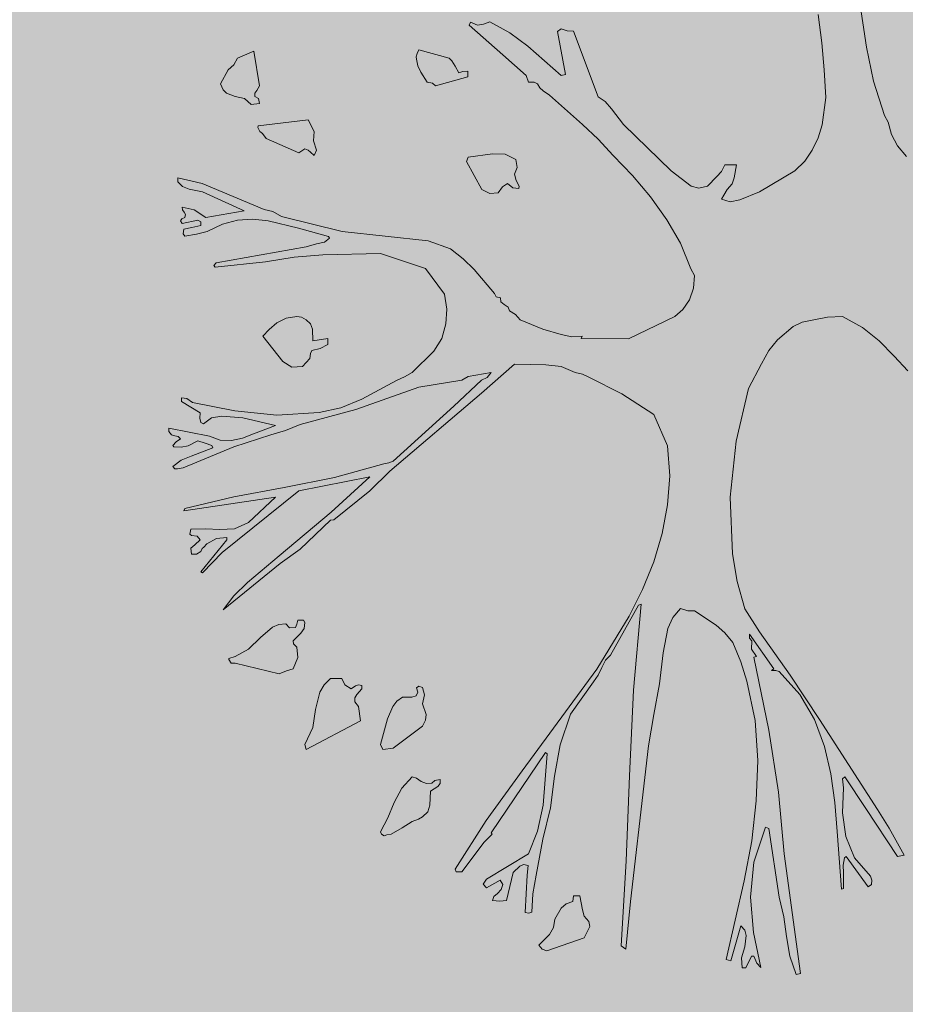
# Model space of a CAD drawing. Units: inches. Extents: x 84 to 1044, y -280 to 906.
# Tile 60 of 105: x 411.62 to 427.1, y 730.84 to 748.06. Entities that reach past the tile are written whole.
import ezdxf

# ---------------------------------------------------------------- set-up
doc = ezdxf.new("R2010")
doc.units = ezdxf.units.IN
doc.layers.add('A-ANNO-DIMS', color=2, linetype='Continuous', lineweight=18)
doc.layers.add('L-PLNT', color=114, linetype='Continuous', lineweight=15)
doc.layers.add('L-PLNT-PATT', color=9, linetype='Continuous', lineweight=9, true_color=0xafd9aa)
doc.styles.get("Standard").update_dxf_attribs({"font": 'arial.ttf'})
doc.dimstyles.get("Standard").update_dxf_attribs({"dimtxt": 0.18, "dimasz": 0.18, "dimexe": 0.18, "dimexo": 0.0625, "dimgap": 0.09, "dimtad": 0, "dimtih": 1, "dimtoh": 1, "dimdec": 4, "dimzin": 0, "dimdsep": 46, "dimtxsty": 'Standard', "dimcen": 0.09, "dimadec": 0, "dimazin": 0, "dimtfac": 1, "dimtdec": 4, "dimtofl": 0, "dimtmove": 0, "dimatfit": 3, "dimfxl": 1, "dimtolj": 1, "dimtzin": 0, "dimarcsym": 0})

# ---------------------------------------------------------------- blocks, each defined once
blk = doc.blocks.new('A$C37E508DF')
for p, q in [((0.7911, 1.1436), (0.8027, 1.0677)), ((0.7512, 1.0728), (0.7469, 1.1054)), ((0.3456, 1.093), (0.3469, 1.0964)), ((0.3842, 1.0591), (0.3456, 1.093)), ((0.3469, 1.0964), (0.355, 1.093)), ((0.355, 1.093), (0.3619, 1.0943)), ((0.3619, 1.0943), (0.3692, 1.0968)), ((0.3692, 1.0968), (0.3923, 1.0844)), ((0.4472, 1.0857), (0.4515, 1.0887)), ((0.4515, 1.0887), (0.4584, 1.0865)), ((0.3923, 1.0844), (0.4129, 1.069)), ((0.4562, 1.0364), (0.4472, 1.0857)), ((0.4584, 1.0865), (0.4657, 1.0861)), ((0.4657, 1.0861), (0.4939, 1.0107)), ((0.4129, 1.069), (0.4515, 1.0351)), ((0.7538, 1.0415), (0.7512, 1.0728)), ((0.8027, 1.0677), (0.8108, 1.0287)), ((0.0746, 1.0475), (0.0789, 1.0552)), ((0.0789, 1.0552), (0.0978, 1.063)), ((0.0978, 1.063), (0.1042, 1.0231)), ((0.2847, 1.0565), (0.2856, 1.0604)), ((0.2851, 1.054), (0.2847, 1.0565)), ((0.2856, 1.0604), (0.2877, 1.0647)), ((0.2877, 1.0647), (0.3224, 1.0552)), ((0.3224, 1.0552), (0.3255, 1.0522)), ((0.4112, 1.0351), (0.3842, 1.0591)), ((0.0682, 1.0415), (0.0746, 1.0475)), ((0.2864, 1.0463), (0.2851, 1.054)), ((0.2899, 1.039), (0.2864, 1.0463)), ((0.3255, 1.0522), (0.3293, 1.0458)), ((0.3293, 1.0458), (0.3336, 1.0381)), ((0.0596, 1.0257), (0.0682, 1.0415)), ((0.2972, 1.0274), (0.2899, 1.039)), ((0.3439, 1.0338), (0.3066, 1.0231)), ((0.3336, 1.0381), (0.3383, 1.0398)), ((0.3383, 1.0398), (0.3439, 1.0402)), ((0.3439, 1.0402), (0.3439, 1.0338)), ((0.4138, 1.0274), (0.4112, 1.0351)), ((0.4515, 1.0351), (0.4562, 1.0364)), ((0.7559, 1.0098), (0.7538, 1.0415)), ((0.0626, 1.0188), (0.0596, 1.0257)), ((0.1042, 1.0231), (0.1012, 1.018)), ((0.3032, 1.0265), (0.2972, 1.0274)), ((0.3066, 1.0231), (0.3032, 1.0265)), ((0.4202, 1.0274), (0.4138, 1.0274)), ((0.4241, 1.0257), (0.4202, 1.0274)), ((0.4267, 1.0209), (0.4241, 1.0257)), ((0.4305, 1.0175), (0.4267, 1.0209)), ((0.8108, 1.0287), (0.8233, 0.9892)), ((0.0665, 1.0149), (0.0626, 1.0188)), ((0.0763, 1.0111), (0.0665, 1.0149)), ((0.087, 1.0085), (0.0763, 1.0111)), ((0.1012, 1.018), (0.099, 1.0149)), ((0.099, 1.0149), (0.099, 1.0111)), ((0.099, 1.0111), (0.1033, 1.0085)), ((0.4378, 1.0124), (0.4305, 1.0175)), ((0.476, 0.9789), (0.4378, 1.0124)), ((0.4939, 1.0107), (0.5021, 1.0051)), ((0.7516, 0.9785), (0.7559, 1.0098)), ((0.0948, 1.0016), (0.087, 1.0085)), ((0.1042, 1.0029), (0.0948, 1.0016)), ((0.1033, 1.0085), (0.1042, 1.0029)), ((0.5021, 1.0051), (0.5094, 0.9969)), ((0.5094, 0.9969), (0.5231, 0.9789)), ((0.8233, 0.9892), (0.8275, 0.9815)), ((0.1025, 0.9751), (0.1029, 0.9772)), ((0.1046, 0.9708), (0.1025, 0.9751)), ((0.1029, 0.9772), (0.1604, 0.9841)), ((0.1604, 0.9841), (0.1672, 0.9708)), ((0.4939, 0.9618), (0.476, 0.9789)), ((0.5231, 0.9789), (0.578, 0.9253)), ((0.7469, 0.9635), (0.7516, 0.9785)), ((0.8275, 0.9815), (0.8314, 0.9673)), ((0.1076, 0.9682), (0.1046, 0.9708)), ((0.1119, 0.9626), (0.1076, 0.9682)), ((0.1672, 0.9708), (0.1664, 0.9601)), ((0.8314, 0.9673), (0.8383, 0.954)), ((0.1496, 0.9463), (0.1119, 0.9626)), ((0.1664, 0.9601), (0.1698, 0.9493)), ((0.5111, 0.9429), (0.4939, 0.9618)), ((0.7401, 0.9493), (0.7469, 0.9635)), ((0.8383, 0.954), (0.8486, 0.942)), ((0.1565, 0.9506), (0.1496, 0.9463)), ((0.1604, 0.9493), (0.1565, 0.9506)), ((0.1629, 0.9468), (0.1604, 0.9493)), ((0.1672, 0.9429), (0.1629, 0.9468)), ((0.1698, 0.9493), (0.1672, 0.9429)), ((0.3426, 0.936), (0.3443, 0.9412)), ((0.3443, 0.9412), (0.3722, 0.9451)), ((0.3722, 0.9451), (0.3868, 0.9446)), ((0.3868, 0.9446), (0.3992, 0.9386)), ((0.5334, 0.9202), (0.5111, 0.9429)), ((0.7315, 0.9365), (0.7401, 0.9493)), ((0.3602, 0.9039), (0.3426, 0.936)), ((0.3992, 0.9386), (0.4009, 0.9292)), ((0.6359, 0.9245), (0.6397, 0.9322)), ((0.6397, 0.9322), (0.653, 0.9322)), ((0.653, 0.9322), (0.6505, 0.9172)), ((0.7203, 0.9253), (0.7315, 0.9365)), ((0.4009, 0.9292), (0.3975, 0.9215)), ((0.3975, 0.9215), (0.3996, 0.9142)), ((0.554, 0.8953), (0.5334, 0.9202)), ((0.578, 0.9253), (0.6011, 0.9077)), ((0.6196, 0.9077), (0.6303, 0.9189)), ((0.6303, 0.9189), (0.6359, 0.9245)), ((0.6796, 0.9013), (0.7203, 0.9253)), ((0.0103, 0.9129), (0.0103, 0.9172)), ((0.0103, 0.9172), (0.0382, 0.9107)), ((0.0159, 0.9073), (0.0103, 0.9129)), ((0.0232, 0.9043), (0.0159, 0.9073)), ((0.0382, 0.9107), (0.1098, 0.8807)), ((0.3898, 0.9107), (0.3838, 0.9069)), ((0.3958, 0.906), (0.3898, 0.9107)), ((0.3996, 0.9142), (0.4031, 0.9077)), ((0.4031, 0.9077), (0.4026, 0.9052)), ((0.6011, 0.9077), (0.6097, 0.9056)), ((0.6097, 0.9056), (0.6196, 0.9077)), ((0.6479, 0.9103), (0.6423, 0.9039)), ((0.6505, 0.9172), (0.6479, 0.9103)), ((0.0386, 0.9013), (0.0232, 0.9043)), ((0.0866, 0.8794), (0.0386, 0.9013)), ((0.3692, 0.8992), (0.3602, 0.9039)), ((0.379, 0.9), (0.3692, 0.8992)), ((0.3838, 0.9069), (0.379, 0.9)), ((0.4026, 0.9052), (0.3958, 0.906)), ((0.6384, 0.8974), (0.6359, 0.8927)), ((0.6423, 0.9039), (0.6384, 0.8974)), ((0.6569, 0.8919), (0.6796, 0.9013)), ((0.5728, 0.8691), (0.554, 0.8953)), ((0.6359, 0.8927), (0.6457, 0.8897)), ((0.6457, 0.8897), (0.6569, 0.8919)), ((0.0159, 0.8803), (0.0154, 0.8837)), ((0.0154, 0.8837), (0.0292, 0.8803)), ((0.0176, 0.8777), (0.0159, 0.8803)), ((0.0193, 0.8752), (0.0176, 0.8777)), ((0.0184, 0.8717), (0.0193, 0.8752)), ((0.0292, 0.8803), (0.0424, 0.8717)), ((0.0424, 0.8717), (0.0866, 0.8794)), ((0.1098, 0.8807), (0.1196, 0.8786)), ((0.1196, 0.8786), (0.1295, 0.873)), ((0.1295, 0.873), (0.1994, 0.8554)), ((0.0133, 0.8679), (0.015, 0.87)), ((0.0154, 0.8649), (0.0133, 0.8679)), ((0.015, 0.87), (0.0184, 0.8717)), ((0.0334, 0.8687), (0.0154, 0.8649)), ((0.0266, 0.8602), (0.0369, 0.8623)), ((0.0369, 0.8666), (0.0334, 0.8687)), ((0.0369, 0.8623), (0.0369, 0.8666)), ((0.0617, 0.864), (0.0442, 0.8554)), ((0.0789, 0.8687), (0.0617, 0.864)), ((0.0965, 0.8696), (0.0789, 0.8687)), ((0.1141, 0.8679), (0.0965, 0.8696)), ((0.1492, 0.8593), (0.1141, 0.8679)), ((0.5887, 0.8421), (0.5728, 0.8691)), ((0.0163, 0.8529), (0.0171, 0.8584)), ((0.0184, 0.8503), (0.0163, 0.8529)), ((0.0171, 0.8584), (0.0266, 0.8602)), ((0.0317, 0.8524), (0.0184, 0.8503)), ((0.0442, 0.8554), (0.0317, 0.8524)), ((0.1835, 0.8499), (0.1492, 0.8593)), ((0.1994, 0.8554), (0.2984, 0.8447)), ((0.1578, 0.8378), (0.1698, 0.8413)), ((0.1698, 0.8413), (0.1792, 0.8434)), ((0.1792, 0.8434), (0.1848, 0.8477)), ((0.1848, 0.8477), (0.1835, 0.8499)), ((0.2984, 0.8447), (0.3242, 0.8357)), ((0.6007, 0.8125), (0.5887, 0.8421)), ((0.0545, 0.8194), (0.1578, 0.8378)), ((0.1771, 0.8288), (0.1441, 0.8258)), ((0.2436, 0.8301), (0.1771, 0.8288)), ((0.2954, 0.813), (0.2436, 0.8301)), ((0.3242, 0.8357), (0.3387, 0.8241)), ((0.0519, 0.8164), (0.0545, 0.8194)), ((0.0532, 0.8143), (0.0519, 0.8164)), ((0.1111, 0.8207), (0.0532, 0.8143)), ((0.1441, 0.8258), (0.1111, 0.8207)), ((0.3387, 0.8241), (0.3512, 0.8117)), ((0.3173, 0.7834), (0.2954, 0.813)), ((0.3512, 0.8117), (0.3748, 0.7842)), ((0.6046, 0.8048), (0.6007, 0.8125)), ((0.6037, 0.7903), (0.6046, 0.8048)), ((0.3199, 0.7662), (0.3173, 0.7834)), ((0.3748, 0.7842), (0.3765, 0.7804)), ((0.599, 0.777), (0.6037, 0.7903)), ((0.3765, 0.7804), (0.3816, 0.7791)), ((0.3816, 0.7791), (0.382, 0.7744)), ((0.382, 0.7744), (0.3859, 0.7714)), ((0.3859, 0.7714), (0.3902, 0.7684)), ((0.5913, 0.7658), (0.599, 0.777)), ((0.3186, 0.7491), (0.3199, 0.7662)), ((0.3902, 0.7684), (0.3919, 0.7641)), ((0.3919, 0.7641), (0.3988, 0.7598)), ((0.3988, 0.7598), (0.4043, 0.7538)), ((0.5823, 0.7577), (0.5913, 0.7658)), ((0.1153, 0.7427), (0.1244, 0.7504)), ((0.1244, 0.7504), (0.1351, 0.7559)), ((0.1351, 0.7559), (0.1471, 0.7577)), ((0.1471, 0.7577), (0.1527, 0.7568)), ((0.1527, 0.7568), (0.1578, 0.7538)), ((0.1578, 0.7538), (0.1629, 0.7491)), ((0.1629, 0.7491), (0.1651, 0.7431)), ((0.3139, 0.7324), (0.3186, 0.7491)), ((0.4043, 0.7538), (0.4301, 0.7431)), ((0.5287, 0.7319), (0.5823, 0.7577)), ((0.7285, 0.7512), (0.7182, 0.7461)), ((0.7401, 0.7534), (0.7285, 0.7512)), ((0.7577, 0.7568), (0.7401, 0.7534)), ((0.7752, 0.7577), (0.7577, 0.7568)), ((0.798, 0.7452), (0.7752, 0.7577)), ((0.1081, 0.7349), (0.1153, 0.7427)), ((0.1651, 0.7431), (0.1655, 0.7298)), ((0.4301, 0.7431), (0.4515, 0.7371)), ((0.4515, 0.7371), (0.4635, 0.7341)), ((0.7182, 0.7461), (0.7002, 0.7307)), ((0.8173, 0.7298), (0.798, 0.7452)), ((0.1312, 0.7058), (0.1081, 0.7349)), ((0.1655, 0.7298), (0.1831, 0.7324)), ((0.1831, 0.7255), (0.1741, 0.7208)), ((0.1831, 0.7324), (0.1831, 0.7255)), ((0.3049, 0.7178), (0.3139, 0.7324)), ((0.4635, 0.7341), (0.4755, 0.7349)), ((0.4755, 0.7349), (0.4742, 0.7324)), ((0.4742, 0.7324), (0.5287, 0.7319)), ((0.7002, 0.7307), (0.6903, 0.7186)), ((0.8344, 0.7122), (0.8173, 0.7298)), ((0.1629, 0.7152), (0.1621, 0.7092)), ((0.1646, 0.7186), (0.1629, 0.7152)), ((0.1741, 0.7208), (0.1646, 0.7186)), ((0.28, 0.6933), (0.3049, 0.7178)), ((0.6903, 0.7186), (0.6818, 0.7032)), ((0.1415, 0.6994), (0.1312, 0.7058)), ((0.1621, 0.7092), (0.1539, 0.7002)), ((0.6818, 0.7032), (0.6667, 0.6749)), ((0.8503, 0.6951), (0.8344, 0.7122)), ((0.1539, 0.7002), (0.1415, 0.6994)), ((0.271, 0.6882), (0.28, 0.6933)), ((0.3709, 0.6933), (0.3533, 0.6903)), ((0.3975, 0.7028), (0.3598, 0.6693)), ((0.3662, 0.6873), (0.3709, 0.6933)), ((0.4339, 0.7019), (0.3975, 0.7028)), ((0.4515, 0.7002), (0.4339, 0.7019)), ((0.4674, 0.6933), (0.4515, 0.7002)), ((0.476, 0.6912), (0.4674, 0.6933)), ((0.2221, 0.6625), (0.262, 0.6839)), ((0.262, 0.6839), (0.271, 0.6882)), ((0.337, 0.6843), (0.2877, 0.6762)), ((0.328, 0.6543), (0.3598, 0.6843)), ((0.3443, 0.6886), (0.337, 0.6843)), ((0.3533, 0.6903), (0.3443, 0.6886)), ((0.3598, 0.6843), (0.3662, 0.6873)), ((0.4832, 0.6878), (0.476, 0.6912)), ((0.521, 0.6685), (0.4832, 0.6878)), ((0.2877, 0.6762), (0.2152, 0.6505)), ((0.3598, 0.6693), (0.2543, 0.5797)), ((0.6667, 0.6749), (0.6526, 0.614)), ((0.0146, 0.6599), (0.0146, 0.6642)), ((0.0146, 0.6642), (0.0206, 0.6633)), ((0.036, 0.6466), (0.0146, 0.6599)), ((0.0206, 0.6633), (0.0274, 0.6586)), ((0.0274, 0.6586), (0.0759, 0.6492)), ((0.1977, 0.6526), (0.2221, 0.6625)), ((0.5578, 0.6449), (0.521, 0.6685)), ((0.0356, 0.6406), (0.036, 0.6466)), ((0.0759, 0.6492), (0.1244, 0.644)), ((0.1244, 0.644), (0.1728, 0.647)), ((0.2152, 0.6505), (0.1509, 0.6333)), ((0.1728, 0.647), (0.1977, 0.6526)), ((0.2581, 0.5913), (0.328, 0.6543)), ((0.0369, 0.6355), (0.0356, 0.6406)), ((0.0399, 0.6342), (0.0369, 0.6355)), ((0.0489, 0.641), (0.0399, 0.6342)), ((0.0609, 0.6428), (0.0489, 0.641)), ((0.0853, 0.641), (0.0609, 0.6428)), ((0.1226, 0.632), (0.0853, 0.641)), ((0.5737, 0.6089), (0.5578, 0.6449)), ((0, 0.629), (0.0467, 0.62)), ((0, 0.6252), (0, 0.629)), ((0.003, 0.6213), (0, 0.6252)), ((0.0973, 0.6226), (0.1226, 0.632)), ((0.1342, 0.6265), (0.1175, 0.6213)), ((0.1509, 0.6333), (0.1342, 0.6265)), ((0.0069, 0.6204), (0.003, 0.6213)), ((0.0047, 0.6093), (0.0086, 0.6132)), ((0.0107, 0.6196), (0.0069, 0.6204)), ((0.0086, 0.6132), (0.0133, 0.617)), ((0.0133, 0.617), (0.0107, 0.6196)), ((0.0334, 0.6145), (0.0223, 0.6089)), ((0.0416, 0.6119), (0.0334, 0.6145)), ((0.0467, 0.62), (0.0592, 0.6153)), ((0.0592, 0.6153), (0.072, 0.6149)), ((0.072, 0.6149), (0.0849, 0.6175)), ((0.1175, 0.6213), (0.0746, 0.6076)), ((0.0849, 0.6175), (0.0973, 0.6226)), ((0.6526, 0.614), (0.6457, 0.5497)), ((0.0056, 0.6076), (0.0047, 0.6093)), ((0.0141, 0.6072), (0.0056, 0.6076)), ((0.0223, 0.6089), (0.0141, 0.6072)), ((0.0746, 0.6076), (0.0163, 0.5836)), ((0.0257, 0.5969), (0.0506, 0.6063)), ((0.0493, 0.6093), (0.0416, 0.6119)), ((0.0506, 0.6063), (0.0493, 0.6093)), ((0.5763, 0.5741), (0.5737, 0.6089)), ((0.0047, 0.5849), (0.0141, 0.5921)), ((0.0141, 0.5921), (0.0257, 0.5969)), ((0.253, 0.5892), (0.2581, 0.5913)), ((0.0069, 0.5823), (0.0047, 0.5849)), ((0.0099, 0.5823), (0.0069, 0.5823)), ((0.0163, 0.5836), (0.0099, 0.5823)), ((0.1904, 0.5724), (0.2474, 0.5879)), ((0.2543, 0.5797), (0.2311, 0.557)), ((0.2474, 0.5879), (0.253, 0.5892)), ((0.1325, 0.5608), (0.1904, 0.5724)), ((0.2311, 0.5729), (0.1496, 0.557)), ((0.1869, 0.5325), (0.2311, 0.5729)), ((0.5737, 0.5407), (0.5763, 0.5741)), ((0.1496, 0.557), (0.0613, 0.4858)), ((0.0746, 0.5501), (0.1325, 0.5608)), ((0.2311, 0.557), (0.1899, 0.5235)), ((0.1226, 0.5497), (0.0171, 0.5338)), ((0.0184, 0.5368), (0.0746, 0.5501)), ((0.0917, 0.5205), (0.1226, 0.5497)), ((0.6457, 0.5497), (0.6483, 0.4845)), ((0.0171, 0.5338), (0.0184, 0.5368)), ((0.5677, 0.5077), (0.5737, 0.5407)), ((0.1269, 0.482), (0.1869, 0.5325)), ((0.1861, 0.5231), (0.1509, 0.4897)), ((0.1899, 0.5235), (0.1861, 0.5231)), ((0.024, 0.5072), (0.0253, 0.5128)), ((0.0253, 0.5128), (0.042, 0.5133)), ((0.042, 0.5133), (0.0587, 0.5124)), ((0.0587, 0.5124), (0.0755, 0.5133)), ((0.0755, 0.5133), (0.0917, 0.5205)), ((0.0262, 0.5055), (0.024, 0.5072)), ((0.0326, 0.5047), (0.0262, 0.5055)), ((0.03, 0.4948), (0.036, 0.5004)), ((0.036, 0.5004), (0.0326, 0.5047)), ((0.0369, 0.4639), (0.0669, 0.5004)), ((0.0549, 0.5021), (0.0437, 0.4961)), ((0.0669, 0.5034), (0.0549, 0.5021)), ((0.0669, 0.5004), (0.0669, 0.5034)), ((0.5578, 0.4751), (0.5677, 0.5077)), ((0.0253, 0.491), (0.03, 0.4948)), ((0.0262, 0.4841), (0.0253, 0.491)), ((0.0382, 0.4905), (0.0369, 0.4871)), ((0.0403, 0.4922), (0.0382, 0.4905)), ((0.0437, 0.4961), (0.0403, 0.4922)), ((0.1509, 0.4897), (0.1282, 0.4734)), ((0.0317, 0.4841), (0.0262, 0.4841)), ((0.0369, 0.4871), (0.0317, 0.4841)), ((0.0613, 0.4858), (0.0386, 0.4627)), ((0.0905, 0.4515), (0.1269, 0.482)), ((0.6483, 0.4845), (0.6539, 0.4524)), ((0.1282, 0.4734), (0.0626, 0.4198)), ((0.545, 0.4434), (0.5578, 0.4751)), ((0.0386, 0.4627), (0.0369, 0.4639)), ((0.0746, 0.4361), (0.0905, 0.4515)), ((0.5295, 0.4125), (0.545, 0.4434)), ((0.6539, 0.4524), (0.6625, 0.4211)), ((0.0626, 0.4198), (0.0746, 0.4361)), ((0.5403, 0.4254), (0.5081, 0.3679)), ((0.5347, 0.3276), (0.5433, 0.4266)), ((0.5433, 0.4266), (0.5403, 0.4254)), ((0.5887, 0.4215), (0.5797, 0.4112)), ((0.5969, 0.4189), (0.5887, 0.4215)), ((0.6625, 0.4211), (0.6796, 0.3945)), ((0.1471, 0.4035), (0.1484, 0.4082)), ((0.1484, 0.4082), (0.1548, 0.4082)), ((0.1548, 0.4082), (0.1565, 0.4052)), ((0.4922, 0.3516), (0.5295, 0.4125)), ((0.5797, 0.4112), (0.5741, 0.3983)), ((0.6046, 0.4189), (0.5969, 0.4189)), ((0.6295, 0.4022), (0.6046, 0.4189)), ((0.1055, 0.388), (0.1192, 0.4001)), ((0.1192, 0.4001), (0.1265, 0.4031)), ((0.1265, 0.4031), (0.1346, 0.4039)), ((0.1346, 0.4039), (0.1389, 0.3992)), ((0.1389, 0.3992), (0.1458, 0.3996)), ((0.1458, 0.3996), (0.1471, 0.4035)), ((0.1556, 0.3983), (0.1518, 0.3932)), ((0.1565, 0.4052), (0.1556, 0.3983)), ((0.5741, 0.3983), (0.5686, 0.3705)), ((0.6397, 0.3936), (0.6295, 0.4022)), ((0.0917, 0.3748), (0.1055, 0.388)), ((0.1518, 0.3932), (0.1432, 0.3842)), ((0.6487, 0.3825), (0.6397, 0.3936)), ((0.6959, 0.352), (0.668, 0.3919)), ((0.668, 0.3919), (0.668, 0.3872)), ((0.668, 0.3872), (0.6706, 0.3842)), ((0.6796, 0.3945), (0.7148, 0.3447)), ((0.0763, 0.3662), (0.0917, 0.3748)), ((0.1432, 0.3842), (0.1436, 0.3808)), ((0.1436, 0.3808), (0.1471, 0.3769)), ((0.1471, 0.3769), (0.1484, 0.3649)), ((0.6582, 0.3602), (0.6487, 0.3825)), ((0.6706, 0.3842), (0.6702, 0.3748)), ((0.6702, 0.3748), (0.6762, 0.3662)), ((0.069, 0.364), (0.0763, 0.3662)), ((0.069, 0.3627), (0.069, 0.364)), ((0.1484, 0.3649), (0.1432, 0.352)), ((0.5081, 0.3679), (0.5025, 0.3619)), ((0.5686, 0.3705), (0.5643, 0.3349)), ((0.6762, 0.3662), (0.6732, 0.3653)), ((0.6732, 0.3653), (0.6903, 0.2813)), ((0.0716, 0.3585), (0.069, 0.3627)), ((0.0763, 0.3585), (0.0716, 0.3585)), ((0.1269, 0.3464), (0.0763, 0.3585)), ((0.1432, 0.352), (0.1355, 0.3499)), ((0.4065, 0.2345), (0.4922, 0.3516)), ((0.4982, 0.3537), (0.4939, 0.3447)), ((0.5025, 0.3619), (0.4982, 0.3537)), ((0.665, 0.3379), (0.6582, 0.3602)), ((0.6933, 0.3503), (0.6959, 0.352)), ((0.1355, 0.3499), (0.1269, 0.3464)), ((0.1788, 0.3336), (0.1861, 0.3409)), ((0.1861, 0.3409), (0.199, 0.3409)), ((0.199, 0.3409), (0.2024, 0.3336)), ((0.4939, 0.3447), (0.4884, 0.337)), ((0.6985, 0.3503), (0.6933, 0.3503)), ((0.7023, 0.349), (0.6985, 0.3503)), ((0.7259, 0.3224), (0.7023, 0.349)), ((0.7148, 0.3447), (0.7487, 0.2937)), ((0.1737, 0.325), (0.1788, 0.3336)), ((0.2024, 0.3336), (0.2097, 0.3289)), ((0.2097, 0.3289), (0.2148, 0.3323)), ((0.2148, 0.3323), (0.2182, 0.3336)), ((0.2221, 0.3289), (0.2161, 0.3224)), ((0.2182, 0.3336), (0.2221, 0.3327)), ((0.2221, 0.3327), (0.2221, 0.3289)), ((0.2851, 0.3302), (0.2877, 0.3319)), ((0.2864, 0.325), (0.2851, 0.3302)), ((0.2877, 0.3319), (0.292, 0.3306)), ((0.292, 0.3306), (0.2941, 0.322)), ((0.4884, 0.337), (0.4622, 0.2997)), ((0.5643, 0.3349), (0.5578, 0.2993)), ((0.6745, 0.2924), (0.665, 0.3379)), ((0.1689, 0.3053), (0.1737, 0.325)), ((0.2161, 0.3224), (0.214, 0.3186)), ((0.214, 0.3186), (0.214, 0.3139)), ((0.2624, 0.3147), (0.2689, 0.3194)), ((0.2689, 0.3194), (0.2796, 0.3194)), ((0.2796, 0.3194), (0.2847, 0.3211)), ((0.2847, 0.3211), (0.2864, 0.325)), ((0.2941, 0.322), (0.292, 0.3117)), ((0.53, 0.229), (0.5347, 0.3276)), ((0.7427, 0.2937), (0.7259, 0.3224)), ((0.214, 0.3139), (0.2182, 0.3087)), ((0.2182, 0.3087), (0.2204, 0.292)), ((0.2517, 0.2946), (0.2577, 0.3087)), ((0.2577, 0.3087), (0.2624, 0.3147)), ((0.292, 0.3117), (0.2959, 0.2993)), ((0.1655, 0.2843), (0.1689, 0.3053)), ((0.2959, 0.2993), (0.2954, 0.2928)), ((0.4622, 0.2997), (0.4502, 0.2645)), ((0.5578, 0.2993), (0.5518, 0.2633)), ((0.1565, 0.265), (0.1655, 0.2843)), ((0.2204, 0.292), (0.1578, 0.259)), ((0.2436, 0.265), (0.2517, 0.2946)), ((0.292, 0.286), (0.2581, 0.2607)), ((0.2954, 0.2928), (0.292, 0.286)), ((0.6775, 0.2465), (0.6745, 0.2924)), ((0.7542, 0.2628), (0.7427, 0.2937)), ((0.7487, 0.2937), (0.8151, 0.1899)), ((0.6903, 0.2813), (0.7015, 0.2101)), ((0.1578, 0.259), (0.1565, 0.265)), ((0.2461, 0.259), (0.2436, 0.265)), ((0.4502, 0.2645), (0.4438, 0.2285)), ((0.5518, 0.2633), (0.5475, 0.2268)), ((0.7615, 0.2311), (0.7542, 0.2628)), ((0.2581, 0.2607), (0.2461, 0.259)), ((0.4335, 0.2556), (0.3709, 0.1634)), ((0.4305, 0.1951), (0.4352, 0.2543)), ((0.4352, 0.2543), (0.4335, 0.2556)), ((0.6758, 0.2002), (0.6775, 0.2465)), ((0.268, 0.2148), (0.28, 0.2277)), ((0.28, 0.2277), (0.2851, 0.226)), ((0.3649, 0.1775), (0.4065, 0.2345)), ((0.4438, 0.2285), (0.4391, 0.1921)), ((0.5261, 0.1308), (0.53, 0.229)), ((0.5475, 0.2268), (0.5313, 0.084)), ((0.7662, 0.1981), (0.7615, 0.2311)), ((0.7778, 0.2277), (0.7752, 0.2255)), ((0.8018, 0.1912), (0.7778, 0.2277)), ((0.2851, 0.226), (0.2903, 0.2225)), ((0.2903, 0.2225), (0.2963, 0.22)), ((0.2963, 0.22), (0.3027, 0.2204)), ((0.3096, 0.2165), (0.301, 0.211)), ((0.3027, 0.2204), (0.3061, 0.2234)), ((0.3061, 0.2234), (0.3122, 0.2247)), ((0.3122, 0.22), (0.3096, 0.2165)), ((0.3122, 0.2247), (0.3122, 0.22)), ((0.7752, 0.2255), (0.7761, 0.2152)), ((0.2594, 0.1981), (0.268, 0.2148)), ((0.301, 0.211), (0.3002, 0.1951)), ((0.7015, 0.2101), (0.7079, 0.1389)), ((0.7761, 0.2152), (0.7752, 0.1861)), ((0.2521, 0.1805), (0.2594, 0.1981)), ((0.3002, 0.1951), (0.298, 0.1874)), ((0.4241, 0.1651), (0.4305, 0.1951)), ((0.6706, 0.1539), (0.6758, 0.2002)), ((0.7688, 0.1646), (0.7662, 0.1981)), ((0.292, 0.1818), (0.2873, 0.1788)), ((0.298, 0.1874), (0.292, 0.1818)), ((0.4391, 0.1921), (0.4301, 0.1561)), ((0.7752, 0.1861), (0.7787, 0.1591)), ((0.8383, 0.1359), (0.8018, 0.1912)), ((0.8151, 0.1899), (0.8288, 0.1685)), ((0.2436, 0.1642), (0.2521, 0.1805)), ((0.28, 0.1762), (0.2684, 0.1689)), ((0.2873, 0.1788), (0.28, 0.1762)), ((0.3293, 0.1213), (0.3649, 0.1775)), ((0.2448, 0.1616), (0.2436, 0.1642)), ((0.2478, 0.1599), (0.2448, 0.1616)), ((0.2508, 0.1608), (0.2478, 0.1599)), ((0.2556, 0.1616), (0.2508, 0.1608)), ((0.2684, 0.1689), (0.2556, 0.1616)), ((0.3692, 0.1591), (0.3628, 0.1526)), ((0.3718, 0.1616), (0.3692, 0.1591)), ((0.3709, 0.1634), (0.3718, 0.1616)), ((0.4138, 0.1389), (0.4241, 0.1651)), ((0.6865, 0.1698), (0.6732, 0.1295)), ((0.6903, 0.1681), (0.6865, 0.1698)), ((0.7023, 0.0892), (0.6903, 0.1681)), ((0.774, 0.0982), (0.7688, 0.1646)), ((0.7787, 0.1591), (0.789, 0.1346)), ((0.8288, 0.1685), (0.846, 0.1376)), ((0.3628, 0.1526), (0.337, 0.1183)), ((0.4301, 0.1561), (0.4224, 0.1145)), ((0.662, 0.108), (0.6706, 0.1539)), ((0.3653, 0.1098), (0.4138, 0.1389)), ((0.7079, 0.1389), (0.7268, 0.0013)), ((0.846, 0.1376), (0.8383, 0.1359)), ((0.4039, 0.1248), (0.3962, 0.1175)), ((0.4082, 0.1269), (0.4039, 0.1248)), ((0.4134, 0.1256), (0.4082, 0.1269)), ((0.4121, 0.1145), (0.4134, 0.1256)), ((0.5205, 0.033), (0.5261, 0.1308)), ((0.6732, 0.1295), (0.6693, 0.0892)), ((0.7774, 0.1346), (0.7757, 0.1261)), ((0.7757, 0.1261), (0.7761, 0.117)), ((0.7791, 0.1359), (0.7774, 0.1346)), ((0.8044, 0.1012), (0.7791, 0.1359)), ((0.789, 0.1346), (0.8074, 0.1132)), ((0.3306, 0.1183), (0.3293, 0.1213)), ((0.337, 0.1183), (0.3306, 0.1183)), ((0.3962, 0.1175), (0.3885, 0.0853)), ((0.4099, 0.0716), (0.4121, 0.1145)), ((0.4224, 0.1145), (0.4189, 0.093)), ((0.7761, 0.117), (0.7761, 0.099)), ((0.3615, 0.1042), (0.3653, 0.1098)), ((0.3653, 0.0999), (0.3615, 0.1042)), ((0.3812, 0.1089), (0.3653, 0.0999)), ((0.3842, 0.1037), (0.3812, 0.1089)), ((0.3825, 0.0978), (0.3842, 0.1037)), ((0.641, 0.0172), (0.662, 0.108)), ((0.8083, 0.1037), (0.8044, 0.1012)), ((0.8074, 0.1132), (0.8087, 0.1089)), ((0.8087, 0.1089), (0.8083, 0.1037)), ((0.3739, 0.09), (0.3782, 0.0935)), ((0.3782, 0.0935), (0.3825, 0.0978)), ((0.4189, 0.093), (0.4176, 0.072)), ((0.7761, 0.099), (0.774, 0.0982)), ((0.3722, 0.0853), (0.3739, 0.09)), ((0.3808, 0.0845), (0.3722, 0.0853)), ((0.3885, 0.0853), (0.3808, 0.0845)), ((0.4515, 0.0763), (0.4571, 0.0815)), ((0.4571, 0.0815), (0.4648, 0.084)), ((0.4648, 0.084), (0.4657, 0.0905)), ((0.4657, 0.0905), (0.473, 0.0905)), ((0.473, 0.0905), (0.476, 0.0746)), ((0.5313, 0.084), (0.5257, 0.0291)), ((0.6693, 0.0892), (0.6728, 0.0484)), ((0.7075, 0.0665), (0.7023, 0.0892)), ((0.4142, 0.0707), (0.4099, 0.0716)), ((0.4176, 0.072), (0.4142, 0.0707)), ((0.4442, 0.0639), (0.4515, 0.0763)), ((0.476, 0.0746), (0.4777, 0.0673)), ((0.4425, 0.0544), (0.4442, 0.0639)), ((0.4777, 0.0673), (0.4832, 0.0613)), ((0.4832, 0.0613), (0.4845, 0.0553)), ((0.7105, 0.0437), (0.7075, 0.0665)), ((0.4258, 0.0339), (0.4378, 0.0463)), ((0.4378, 0.0463), (0.4425, 0.0544)), ((0.4811, 0.0493), (0.4777, 0.0424)), ((0.4845, 0.0553), (0.4811, 0.0493)), ((0.6582, 0.0562), (0.6466, 0.0159)), ((0.6625, 0.051), (0.6582, 0.0562)), ((0.6642, 0.045), (0.6625, 0.051)), ((0.6728, 0.0484), (0.6809, 0.0082)), ((0.4777, 0.0424), (0.4348, 0.0274)), ((0.6625, 0.0321), (0.6642, 0.045)), ((0.7144, 0.0214), (0.7105, 0.0437)), ((0.4296, 0.0291), (0.4258, 0.0339)), ((0.4348, 0.0274), (0.4296, 0.0291)), ((0.5257, 0.0291), (0.5205, 0.033)), ((0.659, 0.0193), (0.6625, 0.0321)), ((0.6466, 0.0159), (0.641, 0.0172)), ((0.6595, 0.0077), (0.659, 0.0193)), ((0.6702, 0.0214), (0.6637, 0.0077)), ((0.6732, 0.0214), (0.6702, 0.0214)), ((0.6766, 0.0133), (0.6732, 0.0214)), ((0.6809, 0.0082), (0.6766, 0.0133)), ((0.7216, 0), (0.7144, 0.0214)), ((0.6637, 0.0077), (0.6595, 0.0077)), ((0.7268, 0.0013), (0.7216, 0))]:
    blk.add_line(p, q)
blk = doc.blocks.new('*D62')
at = {"layer": 'A-ANNO-DIMS', "color": 0, "lineweight": -2, "transparency": 16777216}
for p, q in [((203.179, 709.183), (203.179, 905.9)), ((896.074, 400.183), (896.074, 905.9)), ((203.359, 905.72), (549.232, 905.72)), ((895.894, 905.72), (550.021, 905.72))]:
    blk.add_line(p, q, dxfattribs=at)
at = {"layer": 'A-ANNO-DIMS', "color": 0, "transparency": 16777216}
for points in [[(203.359, 905.75), (203.359, 905.69), (203.179, 905.72)], [(895.894, 905.75), (895.894, 905.69), (896.074, 905.72)]]:
    blk.add_solid(points, dxfattribs=at)
at = {"layer": 'Defpoints', "color": 0, "transparency": 16777216}
for p in [(896.074, 905.72), (203.179, 709.12), (896.074, 400.12)]:
    blk.add_point(p, dxfattribs=at)
at = {"layer": 'A-ANNO-DIMS', "color": 0, "transparency": 16777216, "insert": (549.627, 905.72), "char_height": 0.18, "attachment_point": 5}
blk.add_mtext('\\A1;692.9', dxfattribs=at)

msp = doc.modelspace()

# ---------------------------------------------------------------- hatches: boundary and pattern name
at = {"layer": 'L-PLNT-PATT', "transparency": 33554597}
h = msp.add_hatch(color=256, dxfattribs=at)
h.dxf.hatch_style = 1
h.paths.add_polyline_path([(434.074, 769.12), (386.074, 769.12), (386.074, 709.12), (434.074, 709.12)])
h.paths.add_polyline_path([(896.074, 847.12), (434.074, 847.12), (434.074, 769.12), (434.074, 709.12), (470.074, 709.12), (506.074, 709.12), (572.074, 709.12), (608.074, 709.12), (698.074, 709.12), (770.074, 709.12), (833.074, 709.12), (896.074, 709.12)])
h.paths.add_polyline_path([(983.074, 847.12), (896.074, 847.12), (896.074, 709.12), (896.074, 547.12), (932.074, 547.12), (983.074, 547.12)])
h.paths.add_polyline_path([(983.074, 547.12), (932.074, 547.12), (932.074, 265.12), (983.074, 265.12)])
h.paths.add_polyline_path([(203.179, 646.12), (203.179, 709.12), (203.179, 745.12), (143.179, 745.12), (143.179, 271.12), (203.179, 271.12), (203.179, 274.12), (203.179, 310.12), (203.179, 574.12)])

# ---------------------------------------------------------------- block references
at = {"layer": 'L-PLNT', "xscale": 15.19586232982809, "yscale": 15.19586232982809, "zscale": 15.19586232982809}
msp.add_blockref('A$C37E508DF', (414.225, 731.356), dxfattribs=at)

# ---------------------------------------------------------------- dimensions: what is measured, and where the dimension line sits
at = {"layer": 'A-ANNO-DIMS'}
dim = msp.add_linear_dim(base=(896.074, 905.72), p1=(203.179, 709.12), p2=(896.074, 400.12), dimstyle='Standard', override={"dimdec": 1, "dimlfac": 1, "dimrnd": 0, "dimzin": 0, "dimdsep": 46, "dimlunit": 2}, dxfattribs=at)
dim.commit()
dim.dimension.update_dxf_attribs({"geometry": '*D62', "text_midpoint": (549.627, 905.72)})

doc.saveas('drawing.dxf')
